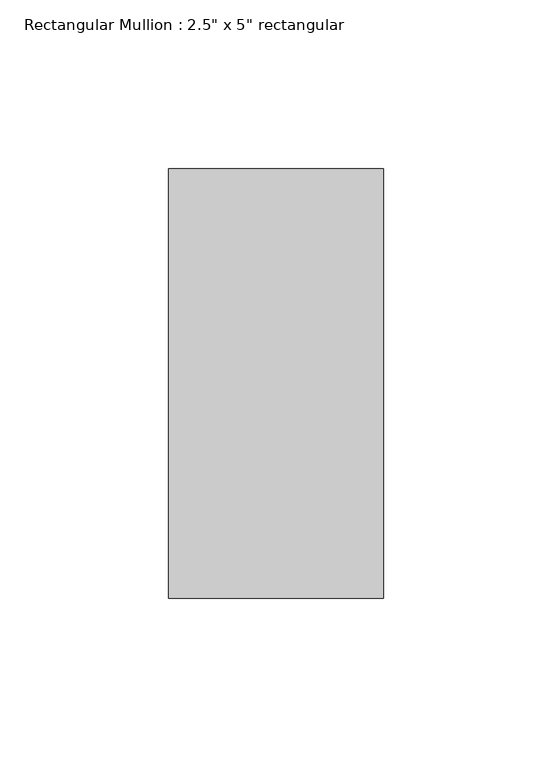
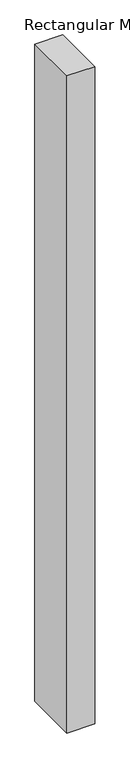
"""IFC4 building model written with IfcOpenShell, lengths in millimetres: member geometry."""

from ifc_helpers import new_model, si_unit, frame, origin, place, context, project, spatial, polyline, outline, extrude, source, transform, mapped, element, save


def member_8d789d2e(model_context):
    return source(origin(), model_context, "Body", "SweptSolid", [
        extrude(outline(polyline([(0.0, 63.5), (0.0, -63.5), (-63.5, -63.5), (-63.5, 63.5), (0.0, 63.5)])), frame((0.0, 0.0, -1587.5291864), z_axis=(0.0, 0.0, 1.0), x_axis=(1.0, 0.0, 0.0)), (0.0, 0.0, 1.0), 1587.5291864),
    ])


if __name__ == "__main__":
    model = new_model("IFC4")
    model_context = context("Model", 3, world=origin())
    ifc_project = project(units=[si_unit("LENGTHUNIT", "METRE", prefix="MILLI")], contexts=[model_context])
    site = spatial("IfcSite", under=ifc_project)
    building = spatial("IfcBuilding", under=site)
    placement = place(None, origin())
    member_shape = member_8d789d2e(model_context)
    element("IfcMember", 1, ObjectType="Rectangular Mullion : 2.5\" x 5\" rectangular", at=placement, inside=building, context=model_context, shape_type="MappedRepresentation", body=[
        mapped(member_shape, transform((0.0, 0.0, 0.0), x_axis=(1.0, 0.0, 0.0), y_axis=(0.0, 1.0, 0.0), z_axis=(0.0, 0.0, 1.0))),
    ])
    save(model, "model.ifc")

# Revit data of these elements
# Type "Rectangular Mullion : 2.5\" x 5\" rectangular"
#   built-in parameter 1007304 = 0.416667 (stored number, unit not read)
#   built-in parameter 1007301 = 0.104167 (stored number, unit not read)
#   built-in parameter 1007300 = 0.104167 (stored number, unit not read)
# Element 1 (IfcMember, "Rectangular Mullion : 2.5\" x 5\" rectangular")
#   Materials on its faces: "Aluminum"
# Materials
#   "Aluminum": class "Metal", colour RGB 247 247 247, transparency 0, Description = "Aluminum 6061", Cost = 0
